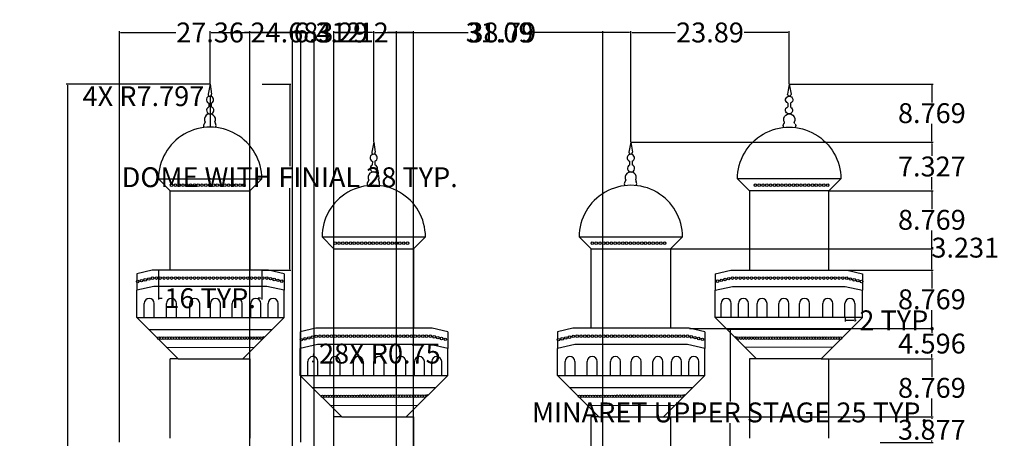
# Model space of a CAD drawing. Units: inches. Extents: x 168 to 318, y 152 to 314.
# Tile 7 of 7: x 170 to 318, y 251 to 314. Entities that reach past the tile are written whole.
import ezdxf

# ---------------------------------------------------------------- set-up
doc = ezdxf.new("R2010")
doc.units = ezdxf.units.IN
doc.header["$MEASUREMENT"] = 0
doc.layers.add('A-ANNO-DIMS', color=2, linetype='Continuous', lineweight=18)
doc.layers.add('A-ELEV', color=7, linetype='Continuous', lineweight=25)
doc.styles.get("Standard").update_dxf_attribs({"font": 'arial.ttf'})
doc.dimstyles.get("Standard").update_dxf_attribs({"dimtxt": 3, "dimasz": 0.18, "dimexe": 0.18, "dimexo": 0.0625, "dimgap": 0.09, "dimtad": 0, "dimtih": 1, "dimtoh": 1, "dimdec": 1, "dimzin": 0, "dimdsep": 46, "dimlunit": 3, "dimtxsty": 'Standard', "dimcen": 0.09, "dimadec": 0, "dimazin": 0, "dimtfac": 1, "dimtdec": 1, "dimtofl": 0, "dimtmove": 0, "dimatfit": 3, "dimfxl": 1, "dimtolj": 1, "dimtzin": 0, "dimarcsym": 0})

# ---------------------------------------------------------------- blocks, each defined once
blk = doc.blocks.new('ARCH-BALCONY-UPPER')
for p, q in [((0, 0), (0, 2.11)), ((1.51, 0), (1.51, 2.11))]:
    blk.add_line(p, q)
blk.add_arc((0.75, 2.11), 0.753, 0, 180)
blk = doc.blocks.new('MINARET-UPPER-STAGE')
for p, q in [((0, 24.84), (0, 22.34)), ((22.23, 24.84), (22.23, 22.34)), ((0, 18.24), (0, 22.34)), ((22.23, 18.24), (22.23, 22.34)), ((6.24, 12), (0, 18.24)), ((0, 18.24), (22.23, 18.24)), ((15.99, 12), (22.23, 18.24)), ((5.07, 0), (5.07, 12)), ((6.24, 12), (5.07, 12)), ((6.24, 12), (15.99, 12)), ((6.24, 12), (15.99, 12)), ((15.99, 12), (17.07, 12)), ((17.07, 12), (17.07, 0))]:
    blk.add_line(p, q)
for points in [[(22.23, 24.84), (19.88, 25.37), (2.34, 25.37), (0, 24.84)], [(22.23, 22.34), (19.61, 22.93), (2.61, 22.93), (0, 22.34)]]:
    blk.add_lwpolyline(points)
blk = doc.blocks.new('DOME-FINIAL')
for p, q in [((198.4, 304.43), (198.12, 302.93)), ((198.4, 304.43), (198.64, 302.93)), ((198.2, 301.56), (198.19, 300.98)), ((198.59, 301.55), (198.59, 301)), ((192.4, 288.34), (190.61, 290.13)), ((190.61, 290.13), (206.2, 290.13)), ((204.4, 288.34), (206.2, 290.13)), ((192.4, 276.34), (192.4, 288.34)), ((192.4, 288.34), (204.4, 288.34)), ((204.4, 288.34), (204.4, 276.34))]:
    blk.add_line(p, q)
for centre, radius, start, end in [((198.4, 302.07), 0.547, 289.437, 247.7441), ((198.38, 302.88), 0.263, 169.3858, 10.6142), ((198.43, 300.48), 0.547, 115.4859, 72.8461), ((197.16, 298.78), 0.5, 317.3553, 349.3337), ((198.38, 299.1), 0.841, 334.1763, 209.1253), ((199.64, 298.73), 0.5, 180, 212.3198), ((198.41, 290.13), 7.8, 0, 180.0146), ((197.83, 298.16), 0.421, 137.3553, 221.1666), ((198.75, 298.17), 0.551, 329.1667, 32.3198)]:
    blk.add_arc(centre, radius, start, end)
blk = doc.blocks.new('*D14')
at = {"layer": 'A-ANNO-DIMS', "color": 0, "lineweight": -2, "ltscale": 0.2, "transparency": 16777216}
for p, q in [((294.19, 269.15), (294.19, 268.6)), ((295.69, 269.15), (295.69, 268.6)), ((294.37, 268.78), (295.51, 268.78)), ((295.69, 268.78), (295.87, 268.78))]:
    blk.add_line(p, q, dxfattribs=at)
at = {"layer": 'A-ANNO-DIMS', "color": 0, "ltscale": 0.2, "transparency": 16777216}
for points in [[(294.37, 268.81), (294.37, 268.75), (294.19, 268.78)], [(295.51, 268.81), (295.51, 268.75), (295.69, 268.78)]]:
    blk.add_solid(points, dxfattribs=at)
at = {"layer": 'Defpoints', "color": 0, "ltscale": 0.2, "transparency": 16777216}
for p in [(294.19, 269.21), (295.69, 269.21), (295.69, 268.78)]:
    blk.add_point(p, dxfattribs=at)
at = {"layer": 'A-ANNO-DIMS', "color": 0, "ltscale": 0.2, "transparency": 16777216, "insert": (302.12, 268.78), "char_height": 3, "attachment_point": 5}
blk.add_mtext('\\A1;2 TYP.', dxfattribs=at)
blk = doc.blocks.new('*D25')
at = {"layer": 'A-ANNO-DIMS', "color": 0, "lineweight": -2, "ltscale": 0.2, "transparency": 16777216}
for p, q in [((273.1, 267.57), (277.02, 267.57)), ((276.84, 267.39), (276.84, 256.52)), ((276.84, 242.38), (276.84, 253.24)), ((273.1, 242.2), (277.02, 242.2))]:
    blk.add_line(p, q, dxfattribs=at)
at = {"layer": 'A-ANNO-DIMS', "color": 0, "ltscale": 0.2, "transparency": 16777216}
for points in [[(276.81, 267.39), (276.87, 267.39), (276.84, 267.57)], [(276.81, 242.38), (276.87, 242.38), (276.84, 242.2)]]:
    blk.add_solid(points, dxfattribs=at)
at = {"layer": 'Defpoints', "color": 0, "ltscale": 0.2, "transparency": 16777216}
for p in [(273.03, 267.57), (276.84, 267.57), (273.03, 242.2)]:
    blk.add_point(p, dxfattribs=at)
at = {"layer": 'A-ANNO-DIMS', "color": 0, "ltscale": 0.2, "transparency": 16777216, "insert": (276.84, 254.88), "char_height": 3, "attachment_point": 5}
blk.add_mtext('\\A1;MINARET UPPER STAGE 25 TYP.', dxfattribs=at)
blk = doc.blocks.new('*D27')
at = {"layer": 'A-ANNO-DIMS', "color": 0, "lineweight": -2, "ltscale": 0.2, "transparency": 16777216}
for p, q in [((206.27, 304.43), (210.6, 304.43)), ((210.42, 304.25), (210.42, 292.03)), ((210.42, 276.52), (210.42, 288.74)), ((206.27, 276.34), (210.6, 276.34))]:
    blk.add_line(p, q, dxfattribs=at)
at = {"layer": 'A-ANNO-DIMS', "color": 0, "ltscale": 0.2, "transparency": 16777216}
for points in [[(210.39, 304.25), (210.45, 304.25), (210.42, 304.43)], [(210.39, 276.52), (210.45, 276.52), (210.42, 276.34)]]:
    blk.add_solid(points, dxfattribs=at)
at = {"layer": 'Defpoints', "color": 0, "ltscale": 0.2, "transparency": 16777216}
for p in [(206.2, 304.43), (210.42, 304.43), (206.2, 276.34)]:
    blk.add_point(p, dxfattribs=at)
at = {"layer": 'A-ANNO-DIMS', "color": 0, "ltscale": 0.2, "transparency": 16777216, "insert": (210.42, 290.38), "char_height": 3, "attachment_point": 5}
blk.add_mtext('\\A1;DOME WITH FINIAL 28 TYP.', dxfattribs=at)
blk = doc.blocks.new('*D28')
at = {"layer": 'A-ANNO-DIMS', "color": 0, "lineweight": -2, "ltscale": 0.2, "transparency": 16777216}
for p, q in [((190.61, 276.27), (190.61, 271.94)), ((206.2, 276.27), (206.2, 271.94)), ((190.79, 272.12), (191.15, 272.12)), ((206.02, 272.12), (205.66, 272.12))]:
    blk.add_line(p, q, dxfattribs=at)
at = {"layer": 'A-ANNO-DIMS', "color": 0, "ltscale": 0.2, "transparency": 16777216}
for points in [[(190.79, 272.15), (190.79, 272.09), (190.61, 272.12)], [(206.02, 272.15), (206.02, 272.09), (206.2, 272.12)]]:
    blk.add_solid(points, dxfattribs=at)
at = {"layer": 'Defpoints', "color": 0, "ltscale": 0.2, "transparency": 16777216}
for p in [(190.61, 276.34), (206.2, 276.34), (206.2, 272.12)]:
    blk.add_point(p, dxfattribs=at)
at = {"layer": 'A-ANNO-DIMS', "color": 0, "ltscale": 0.2, "transparency": 16777216, "insert": (198.41, 272.12), "char_height": 3, "attachment_point": 5}
blk.add_mtext('\\A1;16 TYP.', dxfattribs=at)
blk = doc.blocks.new('*D30')
at = {"layer": 'A-ANNO-DIMS', "color": 0, "lineweight": -2, "ltscale": 0.2, "transparency": 16777216}
for p, q in [((198.4, 304.49), (198.4, 312.41)), ((198.58, 312.23), (204.4, 312.23)), ((222.91, 312.23), (217.09, 312.23)), ((223.09, 295.72), (223.09, 312.41))]:
    blk.add_line(p, q, dxfattribs=at)
at = {"layer": 'A-ANNO-DIMS', "color": 0, "ltscale": 0.2, "transparency": 16777216}
for points in [[(198.58, 312.26), (198.58, 312.2), (198.4, 312.23)], [(222.91, 312.26), (222.91, 312.2), (223.09, 312.23)]]:
    blk.add_solid(points, dxfattribs=at)
at = {"layer": 'Defpoints', "color": 0, "ltscale": 0.2, "transparency": 16777216}
for p in [(223.09, 312.23), (198.4, 304.43), (223.09, 295.66)]:
    blk.add_point(p, dxfattribs=at)
at = {"layer": 'A-ANNO-DIMS', "color": 0, "ltscale": 0.2, "transparency": 16777216, "insert": (210.75, 312.23), "char_height": 3, "attachment_point": 5}
blk.add_mtext('\\A1;24.683', dxfattribs=at)
blk = doc.blocks.new('*D31')
at = {"layer": 'A-ANNO-DIMS', "color": 0, "lineweight": -2, "ltscale": 0.2, "transparency": 16777216}
for p, q in [((223.09, 295.72), (223.09, 312.41)), ((223.27, 312.23), (237.33, 312.23)), ((261.7, 312.23), (247.64, 312.23)), ((261.88, 295.72), (261.88, 312.41))]:
    blk.add_line(p, q, dxfattribs=at)
at = {"layer": 'A-ANNO-DIMS', "color": 0, "ltscale": 0.2, "transparency": 16777216}
for points in [[(223.27, 312.26), (223.27, 312.2), (223.09, 312.23)], [(261.7, 312.26), (261.7, 312.2), (261.88, 312.23)]]:
    blk.add_solid(points, dxfattribs=at)
at = {"layer": 'Defpoints', "color": 0, "ltscale": 0.2, "transparency": 16777216}
for p in [(261.88, 312.23), (223.09, 295.66), (261.88, 295.66)]:
    blk.add_point(p, dxfattribs=at)
at = {"layer": 'A-ANNO-DIMS', "color": 0, "ltscale": 0.2, "transparency": 16777216, "insert": (242.48, 312.23), "char_height": 3, "attachment_point": 5}
blk.add_mtext('\\A1;38.79', dxfattribs=at)
blk = doc.blocks.new('*D32')
at = {"layer": 'A-ANNO-DIMS', "color": 0, "lineweight": -2, "ltscale": 0.2, "transparency": 16777216}
for p, q in [((261.88, 295.72), (261.88, 312.41)), ((262.06, 312.23), (268.64, 312.23)), ((285.58, 312.23), (279, 312.23)), ((285.76, 304.49), (285.76, 312.41))]:
    blk.add_line(p, q, dxfattribs=at)
at = {"layer": 'A-ANNO-DIMS', "color": 0, "ltscale": 0.2, "transparency": 16777216}
for points in [[(262.06, 312.26), (262.06, 312.2), (261.88, 312.23)], [(285.58, 312.26), (285.58, 312.2), (285.76, 312.23)]]:
    blk.add_solid(points, dxfattribs=at)
at = {"layer": 'Defpoints', "color": 0, "ltscale": 0.2, "transparency": 16777216}
for p in [(285.76, 312.23), (285.76, 304.43), (261.88, 295.66)]:
    blk.add_point(p, dxfattribs=at)
at = {"layer": 'A-ANNO-DIMS', "color": 0, "ltscale": 0.2, "transparency": 16777216, "insert": (273.82, 312.23), "char_height": 3, "attachment_point": 5}
blk.add_mtext('\\A1;23.89', dxfattribs=at)
blk = doc.blocks.new('*D33')
at = {"layer": 'A-ANNO-DIMS', "color": 0, "lineweight": -2, "ltscale": 0.2, "transparency": 16777216}
for p, q in [((198.34, 304.43), (176.7, 304.43)), ((176.88, 304.25), (176.88, 234.91)), ((176.88, 162.38), (176.88, 231.72)), ((192.34, 162.2), (176.7, 162.2))]:
    blk.add_line(p, q, dxfattribs=at)
at = {"layer": 'A-ANNO-DIMS', "color": 0, "ltscale": 0.2, "transparency": 16777216}
for points in [[(176.85, 304.25), (176.91, 304.25), (176.88, 304.43)], [(176.85, 162.38), (176.91, 162.38), (176.88, 162.2)]]:
    blk.add_solid(points, dxfattribs=at)
at = {"layer": 'Defpoints', "color": 0, "ltscale": 0.2, "transparency": 16777216}
for p in [(176.88, 304.43), (198.4, 304.43), (192.4, 162.2)]:
    blk.add_point(p, dxfattribs=at)
at = {"layer": 'A-ANNO-DIMS', "color": 0, "ltscale": 0.2, "transparency": 16777216, "insert": (176.88, 233.31), "char_height": 3, "attachment_point": 5}
blk.add_mtext('\\A1;142.24', dxfattribs=at)
blk = doc.blocks.new('*D40')
at = {"layer": 'A-ANNO-DIMS', "color": 0, "lineweight": -2, "ltscale": 0.2, "transparency": 16777216}
for p, q in [((267.94, 254.2), (307.47, 254.2)), ((307.29, 254.02), (307.29, 253.89)), ((299.51, 250.32), (307.47, 250.32)), ((307.29, 250.5), (307.29, 250.64))]:
    blk.add_line(p, q, dxfattribs=at)
at = {"layer": 'A-ANNO-DIMS', "color": 0, "ltscale": 0.2, "transparency": 16777216}
for points in [[(307.26, 254.02), (307.32, 254.02), (307.29, 254.2)], [(307.26, 250.5), (307.32, 250.5), (307.29, 250.32)]]:
    blk.add_solid(points, dxfattribs=at)
at = {"layer": 'Defpoints', "color": 0, "ltscale": 0.2, "transparency": 16777216}
for p in [(267.88, 254.2), (307.29, 254.2), (299.44, 250.32)]:
    blk.add_point(p, dxfattribs=at)
at = {"layer": 'A-ANNO-DIMS', "color": 0, "ltscale": 0.2, "transparency": 16777216, "insert": (307.29, 252.26), "char_height": 3, "attachment_point": 5}
blk.add_mtext('\\A1;3.877', dxfattribs=at)
blk = doc.blocks.new('*D41')
at = {"layer": 'A-ANNO-DIMS', "color": 0, "lineweight": -2, "ltscale": 0.2, "transparency": 16777216}
for p, q in [((291.83, 262.97), (307.47, 262.97)), ((307.29, 262.79), (307.29, 260.21)), ((307.29, 254.38), (307.29, 256.96)), ((267.94, 254.2), (307.47, 254.2))]:
    blk.add_line(p, q, dxfattribs=at)
at = {"layer": 'A-ANNO-DIMS', "color": 0, "ltscale": 0.2, "transparency": 16777216}
for points in [[(307.26, 262.79), (307.32, 262.79), (307.29, 262.97)], [(307.26, 254.38), (307.32, 254.38), (307.29, 254.2)]]:
    blk.add_solid(points, dxfattribs=at)
at = {"layer": 'Defpoints', "color": 0, "ltscale": 0.2, "transparency": 16777216}
for p in [(291.76, 262.97), (307.29, 262.97), (267.88, 254.2)]:
    blk.add_point(p, dxfattribs=at)
at = {"layer": 'A-ANNO-DIMS', "color": 0, "ltscale": 0.2, "transparency": 16777216, "insert": (307.29, 258.59), "char_height": 3, "attachment_point": 5}
blk.add_mtext('\\A1;8.769', dxfattribs=at)
blk = doc.blocks.new('*D42')
at = {"layer": 'A-ANNO-DIMS', "color": 0, "lineweight": -2, "ltscale": 0.2, "transparency": 16777216}
for p, q in [((270.75, 267.57), (307.47, 267.57)), ((307.29, 267.39), (307.29, 266.89)), ((291.83, 262.97), (307.47, 262.97)), ((307.29, 263.15), (307.29, 263.65))]:
    blk.add_line(p, q, dxfattribs=at)
at = {"layer": 'A-ANNO-DIMS', "color": 0, "ltscale": 0.2, "transparency": 16777216}
for points in [[(307.26, 267.39), (307.32, 267.39), (307.29, 267.57)], [(307.26, 263.15), (307.32, 263.15), (307.29, 262.97)]]:
    blk.add_solid(points, dxfattribs=at)
at = {"layer": 'Defpoints', "color": 0, "ltscale": 0.2, "transparency": 16777216}
for p in [(270.69, 267.57), (307.29, 267.57), (291.76, 262.97)]:
    blk.add_point(p, dxfattribs=at)
at = {"layer": 'A-ANNO-DIMS', "color": 0, "ltscale": 0.2, "transparency": 16777216, "insert": (307.29, 265.27), "char_height": 3, "attachment_point": 5}
blk.add_mtext('\\A1;4.596', dxfattribs=at)
blk = doc.blocks.new('*D43')
at = {"layer": 'A-ANNO-DIMS', "color": 0, "lineweight": -2, "ltscale": 0.2, "transparency": 16777216}
for p, q in [((294.56, 276.34), (307.47, 276.34)), ((307.29, 276.16), (307.29, 273.57)), ((307.29, 267.75), (307.29, 270.33)), ((270.75, 267.57), (307.47, 267.57))]:
    blk.add_line(p, q, dxfattribs=at)
at = {"layer": 'A-ANNO-DIMS', "color": 0, "ltscale": 0.2, "transparency": 16777216}
for points in [[(307.26, 276.16), (307.32, 276.16), (307.29, 276.34)], [(307.26, 267.75), (307.32, 267.75), (307.29, 267.57)]]:
    blk.add_solid(points, dxfattribs=at)
at = {"layer": 'Defpoints', "color": 0, "ltscale": 0.2, "transparency": 16777216}
for p in [(294.49, 276.34), (307.29, 276.34), (270.69, 267.57)]:
    blk.add_point(p, dxfattribs=at)
at = {"layer": 'A-ANNO-DIMS', "color": 0, "ltscale": 0.2, "transparency": 16777216, "insert": (307.29, 271.95), "char_height": 3, "attachment_point": 5}
blk.add_mtext('\\A1;8.769', dxfattribs=at)
blk = doc.blocks.new('*D44')
at = {"layer": 'A-ANNO-DIMS', "color": 0, "lineweight": -2, "ltscale": 0.2, "transparency": 16777216}
for p, q in [((267.94, 279.57), (307.47, 279.57)), ((307.29, 279.57), (307.29, 279.75)), ((307.29, 279.75), (307.47, 279.75)), ((307.29, 276.52), (307.29, 279.39)), ((294.56, 276.34), (307.47, 276.34))]:
    blk.add_line(p, q, dxfattribs=at)
at = {"layer": 'A-ANNO-DIMS', "color": 0, "ltscale": 0.2, "transparency": 16777216}
for points in [[(307.26, 279.39), (307.32, 279.39), (307.29, 279.57)], [(307.26, 276.52), (307.32, 276.52), (307.29, 276.34)]]:
    blk.add_solid(points, dxfattribs=at)
at = {"layer": 'Defpoints', "color": 0, "ltscale": 0.2, "transparency": 16777216}
for p in [(267.88, 279.57), (307.29, 279.57), (294.49, 276.34)]:
    blk.add_point(p, dxfattribs=at)
at = {"layer": 'A-ANNO-DIMS', "color": 0, "ltscale": 0.2, "transparency": 16777216, "insert": (312.33, 279.75), "char_height": 3, "attachment_point": 5}
blk.add_mtext('\\A1;3.231', dxfattribs=at)
blk = doc.blocks.new('*D45')
at = {"layer": 'A-ANNO-DIMS', "color": 0, "lineweight": -2, "ltscale": 0.2, "transparency": 16777216}
for p, q in [((291.83, 288.34), (307.47, 288.34)), ((307.29, 288.16), (307.29, 285.57)), ((307.29, 279.75), (307.29, 282.33)), ((267.94, 279.57), (307.47, 279.57))]:
    blk.add_line(p, q, dxfattribs=at)
at = {"layer": 'A-ANNO-DIMS', "color": 0, "ltscale": 0.2, "transparency": 16777216}
for points in [[(307.26, 288.16), (307.32, 288.16), (307.29, 288.34)], [(307.26, 279.75), (307.32, 279.75), (307.29, 279.57)]]:
    blk.add_solid(points, dxfattribs=at)
at = {"layer": 'Defpoints', "color": 0, "ltscale": 0.2, "transparency": 16777216}
for p in [(291.76, 288.34), (307.29, 288.34), (267.88, 279.57)]:
    blk.add_point(p, dxfattribs=at)
at = {"layer": 'A-ANNO-DIMS', "color": 0, "ltscale": 0.2, "transparency": 16777216, "insert": (307.29, 283.95), "char_height": 3, "attachment_point": 5}
blk.add_mtext('\\A1;8.769', dxfattribs=at)
blk = doc.blocks.new('*D46')
at = {"layer": 'A-ANNO-DIMS', "color": 0, "lineweight": -2, "ltscale": 0.2, "transparency": 16777216}
for p, q in [((261.94, 295.66), (307.47, 295.66)), ((307.29, 295.48), (307.29, 293.62)), ((307.29, 288.52), (307.29, 290.38)), ((291.83, 288.34), (307.47, 288.34))]:
    blk.add_line(p, q, dxfattribs=at)
at = {"layer": 'A-ANNO-DIMS', "color": 0, "ltscale": 0.2, "transparency": 16777216}
for points in [[(307.26, 295.48), (307.32, 295.48), (307.29, 295.66)], [(307.26, 288.52), (307.32, 288.52), (307.29, 288.34)]]:
    blk.add_solid(points, dxfattribs=at)
at = {"layer": 'Defpoints', "color": 0, "ltscale": 0.2, "transparency": 16777216}
for p in [(261.88, 295.66), (307.29, 295.66), (291.76, 288.34)]:
    blk.add_point(p, dxfattribs=at)
at = {"layer": 'A-ANNO-DIMS', "color": 0, "ltscale": 0.2, "transparency": 16777216, "insert": (307.29, 292), "char_height": 3, "attachment_point": 5}
blk.add_mtext('\\A1;7.327', dxfattribs=at)
blk = doc.blocks.new('*D47')
at = {"layer": 'A-ANNO-DIMS', "color": 0, "lineweight": -2, "ltscale": 0.2, "transparency": 16777216}
for p, q in [((285.83, 304.43), (307.47, 304.43)), ((307.29, 304.25), (307.29, 301.67)), ((307.29, 295.84), (307.29, 298.42)), ((261.94, 295.66), (307.47, 295.66))]:
    blk.add_line(p, q, dxfattribs=at)
at = {"layer": 'A-ANNO-DIMS', "color": 0, "ltscale": 0.2, "transparency": 16777216}
for points in [[(307.26, 304.25), (307.32, 304.25), (307.29, 304.43)], [(307.26, 295.84), (307.32, 295.84), (307.29, 295.66)]]:
    blk.add_solid(points, dxfattribs=at)
at = {"layer": 'Defpoints', "color": 0, "ltscale": 0.2, "transparency": 16777216}
for p in [(285.76, 304.43), (307.29, 304.43), (261.88, 295.66)]:
    blk.add_point(p, dxfattribs=at)
at = {"layer": 'A-ANNO-DIMS', "color": 0, "ltscale": 0.2, "transparency": 16777216, "insert": (307.29, 300.05), "char_height": 3, "attachment_point": 5}
blk.add_mtext('\\A1;8.769', dxfattribs=at)
blk = doc.blocks.new('*D57')
at = {"layer": 'A-ANNO-DIMS', "color": 0, "lineweight": -2, "ltscale": 0.2, "transparency": 16777216}
for p, q in [((226.54, 195.65), (226.54, 312.41)), ((226.72, 312.23), (236.93, 312.23)), ((257.45, 312.23), (247.24, 312.23)), ((257.63, 195.65), (257.63, 312.41))]:
    blk.add_line(p, q, dxfattribs=at)
at = {"layer": 'A-ANNO-DIMS', "color": 0, "ltscale": 0.2, "transparency": 16777216}
for points in [[(226.72, 312.26), (226.72, 312.2), (226.54, 312.23)], [(257.45, 312.26), (257.45, 312.2), (257.63, 312.23)]]:
    blk.add_solid(points, dxfattribs=at)
at = {"layer": 'Defpoints', "color": 0, "ltscale": 0.2, "transparency": 16777216}
for p in [(257.63, 312.23), (226.54, 195.58), (257.63, 195.58)]:
    blk.add_point(p, dxfattribs=at)
at = {"layer": 'A-ANNO-DIMS', "color": 0, "ltscale": 0.2, "transparency": 16777216, "insert": (242.08, 312.23), "char_height": 3, "attachment_point": 5}
blk.add_mtext('\\A1;31.09', dxfattribs=at)
blk = doc.blocks.new('*D66')
at = {"layer": 'A-ANNO-DIMS', "color": 0, "lineweight": -2, "ltscale": 0.2, "transparency": 16777216}
for p, q in [((184.72, 250.39), (184.72, 312.41)), ((184.9, 312.23), (193.23, 312.23)), ((211.9, 312.23), (203.58, 312.23)), ((212.08, 250.39), (212.08, 312.41))]:
    blk.add_line(p, q, dxfattribs=at)
at = {"layer": 'A-ANNO-DIMS', "color": 0, "ltscale": 0.2, "transparency": 16777216}
for points in [[(184.9, 312.26), (184.9, 312.2), (184.72, 312.23)], [(211.9, 312.26), (211.9, 312.2), (212.08, 312.23)]]:
    blk.add_solid(points, dxfattribs=at)
at = {"layer": 'Defpoints', "color": 0, "ltscale": 0.2, "transparency": 16777216}
for p in [(212.08, 312.23), (184.72, 250.32), (212.08, 250.32)]:
    blk.add_point(p, dxfattribs=at)
at = {"layer": 'A-ANNO-DIMS', "color": 0, "ltscale": 0.2, "transparency": 16777216, "insert": (198.4, 312.23), "char_height": 3, "attachment_point": 5}
blk.add_mtext('\\A1;27.36', dxfattribs=at)
blk = doc.blocks.new('*D67')
at = {"layer": 'A-ANNO-DIMS', "color": 0, "lineweight": -2, "ltscale": 0.2, "transparency": 16777216}
for p, q in [((217.09, 242.26), (217.09, 312.41)), ((217.27, 312.23), (221.01, 312.23)), ((228.91, 312.23), (225.17, 312.23)), ((229.09, 242.26), (229.09, 312.41))]:
    blk.add_line(p, q, dxfattribs=at)
at = {"layer": 'A-ANNO-DIMS', "color": 0, "ltscale": 0.2, "transparency": 16777216}
for points in [[(217.27, 312.26), (217.27, 312.2), (217.09, 312.23)], [(228.91, 312.26), (228.91, 312.2), (229.09, 312.23)]]:
    blk.add_solid(points, dxfattribs=at)
at = {"layer": 'Defpoints', "color": 0, "ltscale": 0.2, "transparency": 16777216}
for p in [(229.09, 312.23), (217.09, 242.2), (229.09, 242.2)]:
    blk.add_point(p, dxfattribs=at)
at = {"layer": 'A-ANNO-DIMS', "color": 0, "ltscale": 0.2, "transparency": 16777216, "insert": (223.09, 312.23), "char_height": 3, "attachment_point": 5}
blk.add_mtext('\\A1;12', dxfattribs=at)
blk = doc.blocks.new('*D82')
at = {"layer": 'A-ANNO-DIMS', "color": 0, "lineweight": -2, "ltscale": 0.2, "transparency": 16777216}
for p, q in [((204.4, 234.58), (204.4, 312.41)), ((204.58, 312.23), (210.64, 312.23)), ((210.82, 238.54), (210.82, 312.41)), ((210.82, 312.23), (211, 312.23))]:
    blk.add_line(p, q, dxfattribs=at)
at = {"layer": 'A-ANNO-DIMS', "color": 0, "ltscale": 0.2, "transparency": 16777216}
for points in [[(204.58, 312.26), (204.58, 312.2), (204.4, 312.23)], [(210.64, 312.26), (210.64, 312.2), (210.82, 312.23)]]:
    blk.add_solid(points, dxfattribs=at)
at = {"layer": 'Defpoints', "color": 0, "ltscale": 0.2, "transparency": 16777216}
for p in [(210.82, 312.23), (210.82, 238.48), (204.4, 234.52)]:
    blk.add_point(p, dxfattribs=at)
at = {"layer": 'A-ANNO-DIMS', "color": 0, "ltscale": 0.2, "transparency": 16777216, "insert": (216.14, 312.23), "char_height": 3, "attachment_point": 5}
blk.add_mtext('\\A1;6.412', dxfattribs=at)
blk = doc.blocks.new('*D83')
at = {"layer": 'A-ANNO-DIMS', "color": 0, "lineweight": -2, "ltscale": 0.2, "transparency": 16777216}
for p, q in [((210.82, 238.54), (210.82, 312.41)), ((211, 312.23), (213.92, 312.23)), ((214.1, 238.54), (214.1, 312.41)), ((214.1, 312.23), (214.28, 312.23))]:
    blk.add_line(p, q, dxfattribs=at)
at = {"layer": 'A-ANNO-DIMS', "color": 0, "ltscale": 0.2, "transparency": 16777216}
for points in [[(211, 312.26), (211, 312.2), (210.82, 312.23)], [(213.92, 312.26), (213.92, 312.2), (214.1, 312.23)]]:
    blk.add_solid(points, dxfattribs=at)
at = {"layer": 'Defpoints', "color": 0, "ltscale": 0.2, "transparency": 16777216}
for p in [(214.1, 312.23), (210.82, 238.48), (214.1, 238.48)]:
    blk.add_point(p, dxfattribs=at)
at = {"layer": 'A-ANNO-DIMS', "color": 0, "ltscale": 0.2, "transparency": 16777216, "insert": (218.27, 312.23), "char_height": 3, "attachment_point": 5}
blk.add_mtext('\\A1;3.29', dxfattribs=at)
blk = doc.blocks.new('*D95')
at = {"layer": 'A-ANNO-DIMS', "color": 0, "lineweight": -2, "ltscale": 0.2, "transparency": 16777216}
for p, q in [((198.22, 302.61), (198.4, 302.61)), ((198.4, 302.61), (198.4, 298.11)), ((198.32, 290.13), (198.5, 290.13)), ((198.41, 290.04), (198.41, 290.22))]:
    blk.add_line(p, q, dxfattribs=at)
at = {"layer": 'A-ANNO-DIMS', "color": 0, "ltscale": 0.2, "transparency": 16777216}
blk.add_solid([(198.43, 298.11), (198.37, 298.11), (198.4, 297.93)], dxfattribs=at)
at = {"layer": 'Defpoints', "color": 0, "ltscale": 0.2, "transparency": 16777216}
for p in [(198.4, 297.93), (198.41, 290.13)]:
    blk.add_point(p, dxfattribs=at)
at = {"layer": 'A-ANNO-DIMS', "color": 0, "ltscale": 0.2, "transparency": 16777216, "insert": (188.35, 302.61), "char_height": 3, "attachment_point": 5}
blk.add_mtext('\\A1;4X R7.797', dxfattribs=at)
blk = doc.blocks.new('*D96')
at = {"layer": 'A-ANNO-DIMS', "color": 0, "lineweight": -2, "ltscale": 0.2, "transparency": 16777216}
for p, q in [((213.98, 263.76), (213.97, 263.49)), ((214.16, 263.76), (213.98, 263.76)), ((213.82, 262.56), (214, 262.56)), ((213.91, 262.47), (213.91, 262.65))]:
    blk.add_line(p, q, dxfattribs=at)
at = {"layer": 'A-ANNO-DIMS', "color": 0, "ltscale": 0.2, "transparency": 16777216}
blk.add_solid([(213.94, 263.49), (214, 263.49), (213.96, 263.31)], dxfattribs=at)
at = {"layer": 'Defpoints', "color": 0, "ltscale": 0.2, "transparency": 16777216}
for p in [(213.96, 263.31), (213.91, 262.56)]:
    blk.add_point(p, dxfattribs=at)
at = {"layer": 'A-ANNO-DIMS', "color": 0, "ltscale": 0.2, "transparency": 16777216, "insert": (224.01, 263.76), "char_height": 3, "attachment_point": 5}
blk.add_mtext('\\A1;28X R0.75', dxfattribs=at)

msp = doc.modelspace()

# ---------------------------------------------------------------- linework, layer by layer
at = {"layer": 'A-ELEV'}
for p, q in [((189.1422, 267.4002), (207.7394, 267.387)), ((295.0267, 267.4002), (276.4296, 267.387)), ((191.794, 264.7484), (205.0341, 264.6817)), ((292.375, 264.7484), (279.1348, 264.6817)), ((213.8256, 258.6314), (232.4228, 258.6182)), ((252.6143, 258.6314), (271.2115, 258.6182)), ((216.4774, 255.9797), (229.7175, 255.913)), ((255.2661, 255.9797), (268.5063, 255.913))]:
    msp.add_line(p, q, dxfattribs=at)
for centre in [(192.5965, 289.1877), (193.1705, 289.1877), (193.7444, 289.1877), (194.3183, 289.1877), (194.8922, 289.1877), (195.4661, 289.1877), (196.04, 289.1877), (196.6139, 289.1877), (197.1878, 289.1877), (197.7617, 289.1877), (198.3356, 289.1877), (198.9095, 289.1877), (199.4834, 289.1877), (200.0573, 289.1877), (200.6312, 289.1877), (201.2051, 289.1877), (201.779, 289.1877), (202.3529, 289.1877), (202.9268, 289.1877), (203.5008, 289.1877), (280.6682, 289.1877), (281.2421, 289.1877), (281.816, 289.1877), (282.3899, 289.1877), (282.9638, 289.1877), (283.5377, 289.1877), (284.1116, 289.1877), (284.6855, 289.1877), (285.2594, 289.1877), (285.8333, 289.1877), (286.4072, 289.1877), (286.9811, 289.1877), (287.5551, 289.1877), (288.129, 289.1877), (288.7029, 289.1877), (289.2768, 289.1877), (289.8507, 289.1877), (290.4246, 289.1877), (290.9985, 289.1877), (291.5724, 289.1877), (217.2799, 280.419), (217.8538, 280.419), (218.4277, 280.419), (219.0016, 280.419), (219.5756, 280.419), (220.1495, 280.419), (220.7234, 280.419), (221.2973, 280.419), (221.8712, 280.419), (222.4451, 280.419), (223.019, 280.419), (223.5929, 280.419), (224.1668, 280.419), (224.7407, 280.419), (225.3146, 280.419), (225.8885, 280.419), (226.4624, 280.419), (227.0363, 280.419), (227.6102, 280.419), (228.1841, 280.419), (256.0687, 280.419), (256.6426, 280.419), (257.2165, 280.419), (257.7904, 280.419), (258.3643, 280.419), (258.9382, 280.419), (259.5121, 280.419), (260.086, 280.419), (260.6599, 280.419), (261.2338, 280.419), (261.8077, 280.419), (262.3816, 280.419), (262.9555, 280.419), (263.5294, 280.419), (264.1033, 280.419), (264.6772, 280.419), (265.2511, 280.419), (265.8251, 280.419), (266.399, 280.419), (266.9729, 280.419), (187.4878, 274.6391), (188.0478, 274.7645), (188.6078, 274.8899), (189.1679, 275.0152), (189.7279, 275.1406), (190.3091, 275.1581), (190.883, 275.1581), (191.4569, 275.1581), (192.0309, 275.1581), (192.6048, 275.1581), (193.1787, 275.1581), (193.7526, 275.1581), (194.3265, 275.1581), (194.9004, 275.1581), (195.4743, 275.1581), (196.0482, 275.1581), (196.6221, 275.1581), (197.196, 275.1581), (197.7699, 275.1581), (198.3438, 275.1581), (198.9177, 275.1581), (199.4916, 275.1581), (200.0655, 275.1581), (200.6394, 275.1581), (201.2133, 275.1581), (201.7873, 275.1581), (202.3612, 275.1581), (202.9351, 275.1581), (203.509, 275.1581), (204.0829, 275.1581), (204.6568, 275.1581), (205.2307, 275.1581), (205.8046, 275.1581), (206.3785, 275.1581), (206.9524, 275.1581), (207.5247, 275.0595), (208.0848, 274.9344), (208.6449, 274.8093), (209.205, 274.6842), (274.964, 274.6842), (275.5241, 274.8093), (276.0842, 274.9344), (276.6443, 275.0595), (277.2165, 275.1581), (277.7904, 275.1581), (278.3643, 275.1581), (278.9382, 275.1581), (279.5122, 275.1581), (280.0861, 275.1581), (280.66, 275.1581), (281.2339, 275.1581), (281.8078, 275.1581), (282.3817, 275.1581), (282.9556, 275.1581), (283.5295, 275.1581), (284.1034, 275.1581), (284.6773, 275.1581), (285.2512, 275.1581), (285.8251, 275.1581), (286.399, 275.1581), (286.9729, 275.1581), (287.5468, 275.1581), (288.1207, 275.1581), (288.6946, 275.1581), (289.2686, 275.1581), (289.8425, 275.1581), (290.4164, 275.1581), (290.9903, 275.1581), (291.5642, 275.1581), (292.1381, 275.1581), (292.712, 275.1581), (293.2859, 275.1581), (293.8598, 275.1581), (294.441, 275.1406), (295.0011, 275.0152), (295.5611, 274.8899), (296.1211, 274.7645), (296.6812, 274.6391), (190.6557, 266.0779), (191.062, 266.0785), (191.4683, 266.0791), (191.8745, 266.0797), (192.2808, 266.0803), (192.687, 266.0809), (193.0933, 266.0814), (193.4996, 266.082), (193.9058, 266.0826), (194.3121, 266.0832), (194.7183, 266.0838), (195.1246, 266.0843), (195.5309, 266.0849), (195.9371, 266.0855), (196.3434, 266.0861), (196.7496, 266.0867), (197.1559, 266.0873), (197.5622, 266.0878), (197.9684, 266.0884), (198.3747, 266.089), (198.7809, 266.0896), (199.1872, 266.0902), (199.5934, 266.0907), (199.9997, 266.0913), (200.406, 266.0919), (200.8122, 266.0925), (201.2185, 266.0931), (201.6247, 266.0937), (202.031, 266.0942), (202.4373, 266.0948), (202.8435, 266.0954), (203.2498, 266.096), (203.656, 266.0966), (204.0623, 266.0972), (204.4686, 266.0977), (204.8748, 266.0983), (205.2811, 266.0989), (205.6873, 266.0995), (206.0936, 266.1001), (212.1711, 265.8703), (212.7312, 265.9957), (213.2912, 266.1211), (213.8513, 266.2465), (214.4113, 266.3719), (214.9925, 266.3893), (215.5664, 266.3893), (216.1403, 266.3893), (216.7142, 266.3893), (217.2881, 266.3893), (217.8621, 266.3893), (218.436, 266.3893), (219.0099, 266.3893), (219.5838, 266.3893), (220.1577, 266.3893), (220.7316, 266.3893), (221.3055, 266.3893), (221.8794, 266.3893), (222.4533, 266.3893), (223.0272, 266.3893), (223.6011, 266.3893), (224.175, 266.3893), (224.7489, 266.3893), (225.3228, 266.3893), (225.8967, 266.3893), (226.4706, 266.3893), (227.0445, 266.3893), (227.6185, 266.3893), (228.1924, 266.3893), (228.7663, 266.3893), (229.3402, 266.3893), (229.9141, 266.3893), (230.488, 266.3893), (231.0619, 266.3893), (231.6358, 266.3893), (232.2081, 266.2908), (232.7682, 266.1657), (233.3283, 266.0406), (233.8884, 265.9155), (250.9599, 265.8703), (251.5199, 265.9957), (252.0799, 266.1211), (252.64, 266.2465), (253.2, 266.3719), (253.7812, 266.3893), (254.3552, 266.3893), (254.9291, 266.3893), (255.503, 266.3893), (256.0769, 266.3893), (256.6508, 266.3893), (257.2247, 266.3893), (257.7986, 266.3893), (258.3725, 266.3893), (258.9464, 266.3893), (259.5203, 266.3893), (260.0942, 266.3893), (260.6681, 266.3893), (261.242, 266.3893), (261.8159, 266.3893), (262.3898, 266.3893), (262.9637, 266.3893), (263.5376, 266.3893), (264.1116, 266.3893), (264.6855, 266.3893), (265.2594, 266.3893), (265.8333, 266.3893), (266.4072, 266.3893), (266.9811, 266.3893), (267.555, 266.3893), (268.1289, 266.3893), (268.7028, 266.3893), (269.2767, 266.3893), (269.8506, 266.3893), (270.4245, 266.3893), (270.9968, 266.2908), (271.5569, 266.1657), (272.117, 266.0406), (272.6771, 265.9155), (278.0753, 266.1001), (278.4816, 266.0995), (278.8879, 266.0989), (279.2941, 266.0983), (279.7004, 266.0977), (280.1066, 266.0972), (280.5129, 266.0966), (280.9192, 266.096), (281.3254, 266.0954), (281.7317, 266.0948), (282.1379, 266.0942), (282.5442, 266.0937), (282.9505, 266.0931), (283.3567, 266.0925), (283.763, 266.0919), (284.1692, 266.0913), (284.5755, 266.0907), (284.9817, 266.0902), (285.388, 266.0896), (285.7943, 266.089), (286.2005, 266.0884), (286.6068, 266.0878), (287.013, 266.0873), (287.4193, 266.0867), (287.8256, 266.0861), (288.2318, 266.0855), (288.6381, 266.0849), (289.0443, 266.0843), (289.4506, 266.0838), (289.8569, 266.0832), (290.2631, 266.0826), (290.6694, 266.082), (291.0756, 266.0814), (291.4819, 266.0809), (291.8882, 266.0803), (292.2944, 266.0797), (292.7007, 266.0791), (293.1069, 266.0785), (293.5132, 266.0779), (215.3391, 257.3092), (215.7454, 257.3098), (216.1516, 257.3104), (216.5579, 257.3109), (216.9642, 257.3115), (217.3704, 257.3121), (217.7767, 257.3127), (218.1829, 257.3133), (218.5892, 257.3138), (218.9955, 257.3144), (219.4017, 257.315), (219.808, 257.3156), (220.2142, 257.3162), (220.6205, 257.3168), (221.0268, 257.3173), (221.433, 257.3179), (221.8393, 257.3185), (222.2455, 257.3191), (222.6518, 257.3197), (223.0581, 257.3203), (223.4643, 257.3208), (223.8706, 257.3214), (224.2768, 257.322), (224.6831, 257.3226), (225.0894, 257.3232), (225.4956, 257.3237), (225.9019, 257.3243), (226.3081, 257.3249), (226.7144, 257.3255), (227.1207, 257.3261), (227.5269, 257.3267), (227.9332, 257.3272), (228.3394, 257.3278), (228.7457, 257.3284), (229.1519, 257.329), (229.5582, 257.3296), (229.9645, 257.3301), (230.3707, 257.3307), (230.777, 257.3313), (254.1279, 257.3092), (254.5341, 257.3098), (254.9404, 257.3104), (255.3466, 257.3109), (255.7529, 257.3115), (256.1591, 257.3121), (256.5654, 257.3127), (256.9717, 257.3133), (257.3779, 257.3138), (257.7842, 257.3144), (258.1904, 257.315), (258.5967, 257.3156), (259.003, 257.3162), (259.4092, 257.3168), (259.8155, 257.3173), (260.2217, 257.3179), (260.628, 257.3185), (261.0343, 257.3191), (261.4405, 257.3197), (261.8468, 257.3203), (262.253, 257.3208), (262.6593, 257.3214), (263.0656, 257.322), (263.4718, 257.3226), (263.8781, 257.3232), (264.2843, 257.3237), (264.6906, 257.3243), (265.0969, 257.3249), (265.5031, 257.3255), (265.9094, 257.3261), (266.3156, 257.3267), (266.7219, 257.3272), (267.1282, 257.3278), (267.5344, 257.3284), (267.9407, 257.329), (268.3469, 257.3296), (268.7532, 257.3301), (269.1594, 257.3307), (269.5657, 257.3313)]:
    msp.add_circle(centre, 0.1913, dxfattribs=at)
for centre, start, end in [((206.4999, 266.1006), 54.95912, 215.04088), ((277.6691, 266.1006), 324.95912, 125.04088), ((231.1832, 257.3319), 54.95912, 215.04088), ((269.972, 257.3319), 54.95912, 215.04088)]:
    msp.add_arc(centre, 0.1913, start, end, dxfattribs=at)

# ---------------------------------------------------------------- block references
for name, p in [('DOME-FINIAL', (0, 0)), ('DOME-FINIAL', (24.6834, -8.7688)), ('DOME-FINIAL', (63.4721, -8.7688)), ('MINARET-UPPER-STAGE', (187.332, 250.97)), ('ARCH-BALCONY-UPPER', (188.477, 269.21)), ('ARCH-BALCONY-UPPER', (191.8234, 269.21)), ('ARCH-BALCONY-UPPER', (195.3361, 269.21)), ('ARCH-BALCONY-UPPER', (198.447, 269.21)), ('ARCH-BALCONY-UPPER', (201.7444, 269.21)), ('ARCH-BALCONY-UPPER', (204.5451, 269.21)), ('ARCH-BALCONY-UPPER', (207.1559, 269.21)), ('ARCH-BALCONY-UPPER', (275.5069, 269.21)), ('ARCH-BALCONY-UPPER', (278.1177, 269.21)), ('ARCH-BALCONY-UPPER', (280.9184, 269.21)), ('ARCH-BALCONY-UPPER', (284.2158, 269.21)), ('ARCH-BALCONY-UPPER', (287.3267, 269.21)), ('ARCH-BALCONY-UPPER', (290.8394, 269.21)), ('ARCH-BALCONY-UPPER', (294.1858, 269.21)), ('MINARET-UPPER-STAGE', (212.0154, 242.2012)), ('MINARET-UPPER-STAGE', (250.8041, 242.2012)), ('ARCH-BALCONY-UPPER', (213.1604, 260.4412)), ('ARCH-BALCONY-UPPER', (216.5068, 260.4412)), ('ARCH-BALCONY-UPPER', (220.0195, 260.4412)), ('ARCH-BALCONY-UPPER', (223.1304, 260.4412)), ('ARCH-BALCONY-UPPER', (226.4278, 260.4412)), ('ARCH-BALCONY-UPPER', (229.2285, 260.4412)), ('ARCH-BALCONY-UPPER', (231.8393, 260.4412)), ('ARCH-BALCONY-UPPER', (251.9491, 260.4412)), ('ARCH-BALCONY-UPPER', (255.2955, 260.4412)), ('ARCH-BALCONY-UPPER', (258.8082, 260.4412)), ('ARCH-BALCONY-UPPER', (261.9191, 260.4412)), ('ARCH-BALCONY-UPPER', (265.2165, 260.4412)), ('ARCH-BALCONY-UPPER', (268.0172, 260.4412)), ('ARCH-BALCONY-UPPER', (270.628, 260.4412))]:
    msp.add_blockref(name, p, dxfattribs=at)
at = {"layer": 'A-ELEV', "extrusion": (0, 0, -1), "zscale": -1}
for name, p in [('DOME-FINIAL', (-484.1689, 0)), ('MINARET-UPPER-STAGE', (-296.8369, 250.97))]:
    msp.add_blockref(name, p, dxfattribs=at)

# ---------------------------------------------------------------- dimensions: what is measured, and where the dimension line sits
at = {"layer": 'A-ANNO-DIMS', "ltscale": 0.2}
for base, p1, p2, override, picture, middle in [((212.0845, 312.2308), (184.7244, 250.3243), (212.0845, 250.3243), {"dimdec": 2, "dimlfac": 1, "dimrnd": 0, "dimzin": 0, "dimdsep": 46, "dimlunit": 2}, '*D66', (198.4044, 312.2308)), ((223.0878, 312.2308), (198.4044, 304.4308), (223.0878, 295.6621), {"dimdec": 3, "dimlfac": 1, "dimrnd": 0, "dimzin": 0, "dimdsep": 46, "dimlunit": 2}, '*D30', (210.7461, 312.2308)), ((210.8168, 312.2308), (204.4044, 234.5213), (210.8168, 238.4767), {"dimdec": 3, "dimlfac": 1, "dimrnd": 0, "dimzin": 0, "dimdsep": 46, "dimlunit": 2}, '*D82', (216.1414, 312.2308)), ((214.1032, 312.2308), (210.8168, 238.4767), (214.1032, 238.4767), {"dimdec": 2, "dimlfac": 1, "dimrnd": 0, "dimzin": 0, "dimdsep": 46, "dimlunit": 2}, '*D83', (218.2716, 312.2308)), ((229.0878, 312.2308), (217.0878, 242.2013), (229.0878, 242.2013), {"dimdec": 0, "dimlfac": 1, "dimrnd": 0, "dimzin": 0, "dimdsep": 46, "dimlunit": 2}, '*D67', (223.0878, 312.2308)), ((261.8765, 312.2308), (223.0878, 295.6621), (261.8765, 295.6621), {"dimdec": 2, "dimlfac": 1, "dimrnd": 0, "dimzin": 0, "dimdsep": 46, "dimlunit": 2}, '*D31', (242.4822, 312.2308)), ((257.6286, 312.2308), (226.5403, 195.5844), (257.6286, 195.5844), {"dimdec": 2, "dimlfac": 1, "dimrnd": 0, "dimzin": 0, "dimdsep": 46, "dimlunit": 2}, '*D57', (242.0845, 312.2308)), ((285.7645, 312.2308), (261.8765, 295.6621), (285.7645, 304.4308), {"dimdec": 2, "dimlfac": 1, "dimrnd": 0, "dimzin": 0, "dimdsep": 46, "dimlunit": 2}, '*D32', (273.8205, 312.2308))]:
    dim = msp.add_linear_dim(base=base, p1=p1, p2=p2, dimstyle='Standard', override=override, dxfattribs=at)
    dim.commit()
    dim.dimension.update_dxf_attribs({"geometry": picture, "text_midpoint": middle})
for center, mpoint, text, override, picture, middle in [((198.4054, 290.1334), (198.404, 297.9308), '4X <>', {"dimdec": 3, "dimlfac": 1, "dimrnd": 0, "dimzin": 0, "dimdsep": 46, "dimlunit": 2}, '*D95', (188.3525, 302.6092)), ((213.9135, 262.556), (213.9561, 263.3075), '28X <>', {"dimdec": 2, "dimlfac": 1, "dimrnd": 0, "dimzin": 0, "dimdsep": 46, "dimlunit": 2}, '*D96', (224.0088, 263.7584))]:
    dim = msp.add_radius_dim(center=center, mpoint=mpoint, text=text, dimstyle='Standard', override=override, dxfattribs=at)
    dim.commit()
    dim.dimension.update_dxf_attribs({"geometry": picture, "text_midpoint": middle, "dimtype": 164})
for base, p1, p2, override, picture, middle in [((176.8805, 304.4308), (192.4044, 162.1954), (198.4044, 304.4308), {"dimdec": 2, "dimlfac": 1, "dimrnd": 0, "dimzin": 0, "dimdsep": 46, "dimlunit": 2}, '*D33', (176.8805, 233.3131)), ((307.2884, 304.4308), (261.8765, 295.6621), (285.7645, 304.4308), {"dimdec": 3, "dimlfac": 1, "dimrnd": 0, "dimzin": 0, "dimdsep": 46, "dimlunit": 2}, '*D47', (307.2884, 300.0464)), ((307.2884, 295.6621), (291.7645, 288.3351), (261.8765, 295.6621), {"dimdec": 3, "dimlfac": 1, "dimrnd": 0, "dimzin": 0, "dimdsep": 46, "dimlunit": 2}, '*D46', (307.2884, 291.9986)), ((307.2884, 288.3351), (267.8765, 279.5663), (291.7645, 288.3351), {"dimdec": 3, "dimlfac": 1, "dimrnd": 0, "dimzin": 0, "dimdsep": 46, "dimlunit": 2}, '*D45', (307.2884, 283.9507)), ((307.2884, 279.5663), (294.4933, 276.3351), (267.8765, 279.5663), {"dimdec": 3, "dimlfac": 1, "dimrnd": 0, "dimzin": 0, "dimdsep": 46, "dimlunit": 2}, '*D44', (312.3296, 279.7463)), ((307.2884, 276.3351), (270.6854, 267.5663), (294.4933, 276.3351), {"dimdec": 3, "dimlfac": 1, "dimrnd": 0, "dimzin": 0, "dimdsep": 46, "dimlunit": 2}, '*D43', (307.2884, 271.9507)), ((307.2884, 267.5663), (291.7645, 262.9701), (270.6854, 267.5663), {"dimdec": 3, "dimlfac": 1, "dimrnd": 0, "dimzin": 0, "dimdsep": 46, "dimlunit": 2}, '*D42', (307.2884, 265.2682)), ((307.2884, 262.9701), (267.8765, 254.2013), (291.7645, 262.9701), {"dimdec": 3, "dimlfac": 1, "dimrnd": 0, "dimzin": 0, "dimdsep": 46, "dimlunit": 2}, '*D41', (307.2884, 258.5857)), ((307.2884, 254.2013), (299.4446, 250.3243), (267.8765, 254.2013), {"dimdec": 3, "dimlfac": 1, "dimrnd": 0, "dimzin": 0, "dimdsep": 46, "dimlunit": 2}, '*D40', (307.2884, 252.2628))]:
    dim = msp.add_linear_dim(base=base, p1=p1, p2=p2, angle=90, dimstyle='Standard', override=override, dxfattribs=at)
    dim.commit()
    dim.dimension.update_dxf_attribs({"geometry": picture, "text_midpoint": middle})
for base, p1, p2, text, picture, middle in [((210.4172, 304.4308), (206.2028, 276.3351), (206.2028, 304.4308), 'DOME WITH FINIAL <> TYP.', '*D27', (210.4172, 290.3829)), ((276.8396, 267.5663), (273.0348, 242.2013), (273.0348, 267.5663), 'MINARET UPPER STAGE <> TYP.', '*D25', (276.8396, 254.8838))]:
    dim = msp.add_linear_dim(base=base, p1=p1, p2=p2, angle=90, text=text, dimstyle='Standard', override={"dimdec": 0, "dimrnd": 0, "dimzin": 0, "dimlunit": 2}, dxfattribs=at)
    dim.commit()
    dim.dimension.update_dxf_attribs({"geometry": picture, "text_midpoint": middle})
for base, p1, p2, picture, middle in [((206.2028, 272.1207), (190.6073, 276.3351), (206.2028, 276.3351), '*D28', (198.4051, 272.1207)), ((295.6916, 268.7802), (294.1862, 269.2103), (295.6916, 269.2103), '*D14', (302.1232, 268.7802))]:
    dim = msp.add_linear_dim(base=base, p1=p1, p2=p2, text='<> TYP.', dimstyle='Standard', override={"dimdec": 0, "dimrnd": 0, "dimzin": 0, "dimlunit": 2}, dxfattribs=at)
    dim.commit()
    dim.dimension.update_dxf_attribs({"geometry": picture, "text_midpoint": middle})

doc.saveas('drawing.dxf')
